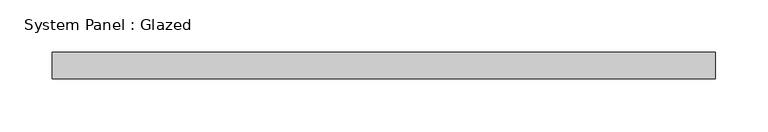
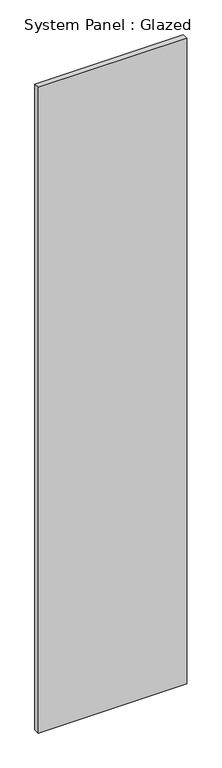
"""IFC4 building model written with IfcOpenShell, lengths in millimetres: plate geometry, System Panel : Glazed."""

from ifc_helpers import new_model, si_unit, origin, origin_with_axes, place, context, project, spatial, polyline, outline, extrude, source, transform, mapped, element, save


def system_panel_glazed_14fb9695(model_context):
    return source(origin(), model_context, "Body", "SweptSolid", [
        extrude(outline(polyline([(317.5, 19.05), (-317.5, 19.05), (-317.5, 44.45), (317.5, 44.45), (317.5, 19.05)])), origin_with_axes(), (0.0, 0.0, 1.0), 2921.0),
    ])


if __name__ == "__main__":
    model = new_model("IFC4")
    model_context = context("Model", 3, world=origin())
    ifc_project = project(units=[si_unit("LENGTHUNIT", "METRE", prefix="MILLI")], contexts=[model_context])
    site = spatial("IfcSite", under=ifc_project)
    building = spatial("IfcBuilding", under=site)
    placement = place(None, origin())
    system_panel_glazed_shape = system_panel_glazed_14fb9695(model_context)
    element("IfcPlate", 1, ObjectType="System Panel : Glazed", at=placement, inside=building, context=model_context, shape_type="MappedRepresentation", body=[
        mapped(system_panel_glazed_shape, transform((0.0, 0.0, 0.0), x_axis=(1.0, 0.0, 0.0), y_axis=(0.0, 1.0, 0.0), z_axis=(0.0, 0.0, 1.0))),
    ])
    save(model, "model.ifc")

# Revit data of these elements
# Type "System Panel : Glazed"
#   Construction Type Id = "GSP4R"
#   Analytic Construction = "1/8 in Pilkington single glazing"
#   Visual Light Transmittance = 0.9
#   Solar Heat Gain Coefficient = 0.86
#   Heat Transfer Coefficient (U) = 1.18115 BTU/(h·ft²·°F)
# Element 1 (IfcPlate, "System Panel : Glazed")
#   Materials on its faces: "Glass"
# Materials
#   "Glass": class "Glass", colour RGB 0 128 192, transparency 0.75, Description = "Soda Lime Glass", Cost = 0
